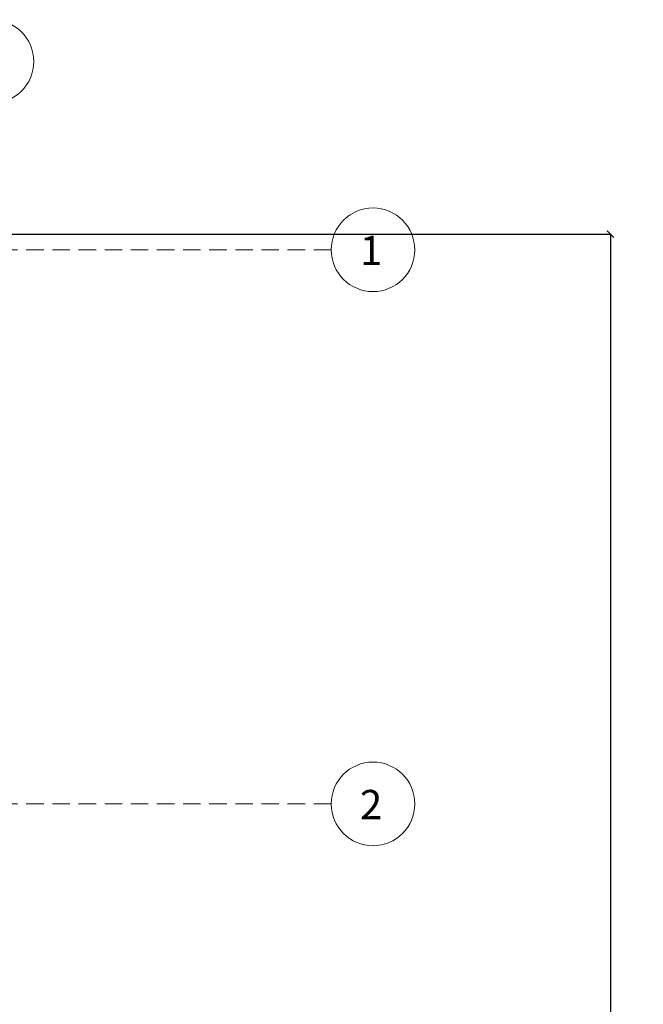
# Model space of a CAD drawing. Units: inches. Extents: x 782 to 2660, y -1008 to 166.
# Tile 11 of 12: x 1410 to 1589, y -176 to 107. Entities that reach past the tile are written whole.
import ezdxf

# ---------------------------------------------------------------- set-up
doc = ezdxf.new("R2010")
doc.units = ezdxf.units.IN
doc.header["$MEASUREMENT"] = 0
doc.linetypes.add('DASHED', pattern=[0.75, 0.5, -0.25])
for name, color, linetype, lineweight in [('A-ANNO-DIMS', 4, 'Continuous', 18), ('A-GRID', 8, 'DASHED', 13), ('A-GRID-IDEN', 7, 'Continuous', 18)]:
    doc.layers.add(name, color=color, linetype=linetype, lineweight=lineweight)
doc.styles.get("Standard").update_dxf_attribs({"font": 'arial.ttf'})
doc.dimstyles.get("Standard").update_dxf_attribs({"dimtxt": 5, "dimasz": 2, "dimexe": 0.18, "dimexo": 0.0625, "dimgap": 0.09, "dimtad": 0, "dimtih": 1, "dimtoh": 1, "dimdec": 0, "dimzin": 0, "dimdsep": 46, "dimlunit": 3, "dimtxsty": 'Standard', "dimblk": 'ARCHTICK', "dimcen": 0.09, "dimadec": 0, "dimazin": 0, "dimtfac": 1, "dimtdec": 0, "dimtofl": 0, "dimtmove": 0, "dimatfit": 3, "dimfxl": 1, "dimtolj": 1, "dimtzin": 0, "dimarcsym": 0})

# ---------------------------------------------------------------- blocks, each defined once
blk = doc.blocks.new('_ArchTick')
at = {"color": 0, "linetype": 'ByBlock', "const_width": 0.15}
blk.add_lwpolyline([(-0.5, -0.5), (0.5, 0.5)], dxfattribs=at)
blk = doc.blocks.new('*D51')
at = {"layer": 'A-ANNO-DIMS', "color": 0, "lineweight": -2, "transparency": 16777216}
for p, q in [((1406.75, 45.01), (1579.89, 45.01)), ((1579.71, 45.01), (1579.71, -327.35)), ((1579.71, -704.99), (1579.71, -332.64)), ((1406.75, -704.99), (1579.89, -704.99))]:
    blk.add_line(p, q, dxfattribs=at)
at = {"layer": 'Defpoints', "color": 0, "transparency": 16777216}
for p in [(1406.68, 45.01), (1579.71, 45.01), (1406.68, -704.99)]:
    blk.add_point(p, dxfattribs=at)
at = {"layer": 'A-ANNO-DIMS', "color": 0, "lineweight": -2, "transparency": 16777216, "xscale": 2, "yscale": 2, "zscale": 2}
for p, rotation in [((1579.71, 45.01), 90), ((1579.71, -704.99), 270)]:
    blk.add_blockref('_ArchTick', p, dxfattribs=dict(at, rotation=rotation))
at = {"layer": 'A-ANNO-DIMS', "color": 0, "transparency": 16777216, "insert": (1579.71, -329.99), "char_height": 5, "attachment_point": 5}
blk.add_mtext('\\A1;62\'-6"', dxfattribs=at)

msp = doc.modelspace()

# ---------------------------------------------------------------- linework, layer by layer
at = {"layer": 'A-GRID', "ltscale": 10}
for p, q in [((1499.56, 40.51), (955.26, 40.51)), ((1499.56, -118.49), (876.32, -118.49))]:
    msp.add_line(p, q, dxfattribs=at)
at = {"layer": 'A-GRID-IDEN'}
for centre in [(1402.18, 94.53), (1511.56, 40.51), (1511.56, -118.49)]:
    msp.add_circle(centre, 12, dxfattribs=at)

# ---------------------------------------------------------------- texts
for s, p in [('1', (1507.82, 36.11)), ('2', (1507.82, -122.89))]:
    msp.add_text(s, height=8.41, dxfattribs=at).set_placement(p)

# ---------------------------------------------------------------- dimensions: what is measured, and where the dimension line sits
at = {"layer": 'A-ANNO-DIMS'}
dim = msp.add_linear_dim(base=(1579.71, 45.01), p1=(1406.68, -704.99), p2=(1406.68, 45.01), angle=90, dimstyle='Standard', override={"dimdec": 1, "dimlfac": 1, "dimrnd": 0, "dimzin": 1, "dimdsep": 46, "dimlunit": 4, "dimfrac": 2}, dxfattribs=at)
dim.commit()
dim.dimension.update_dxf_attribs({"geometry": '*D51', "text_midpoint": (1579.71, -329.99)})

doc.saveas('drawing.dxf')
